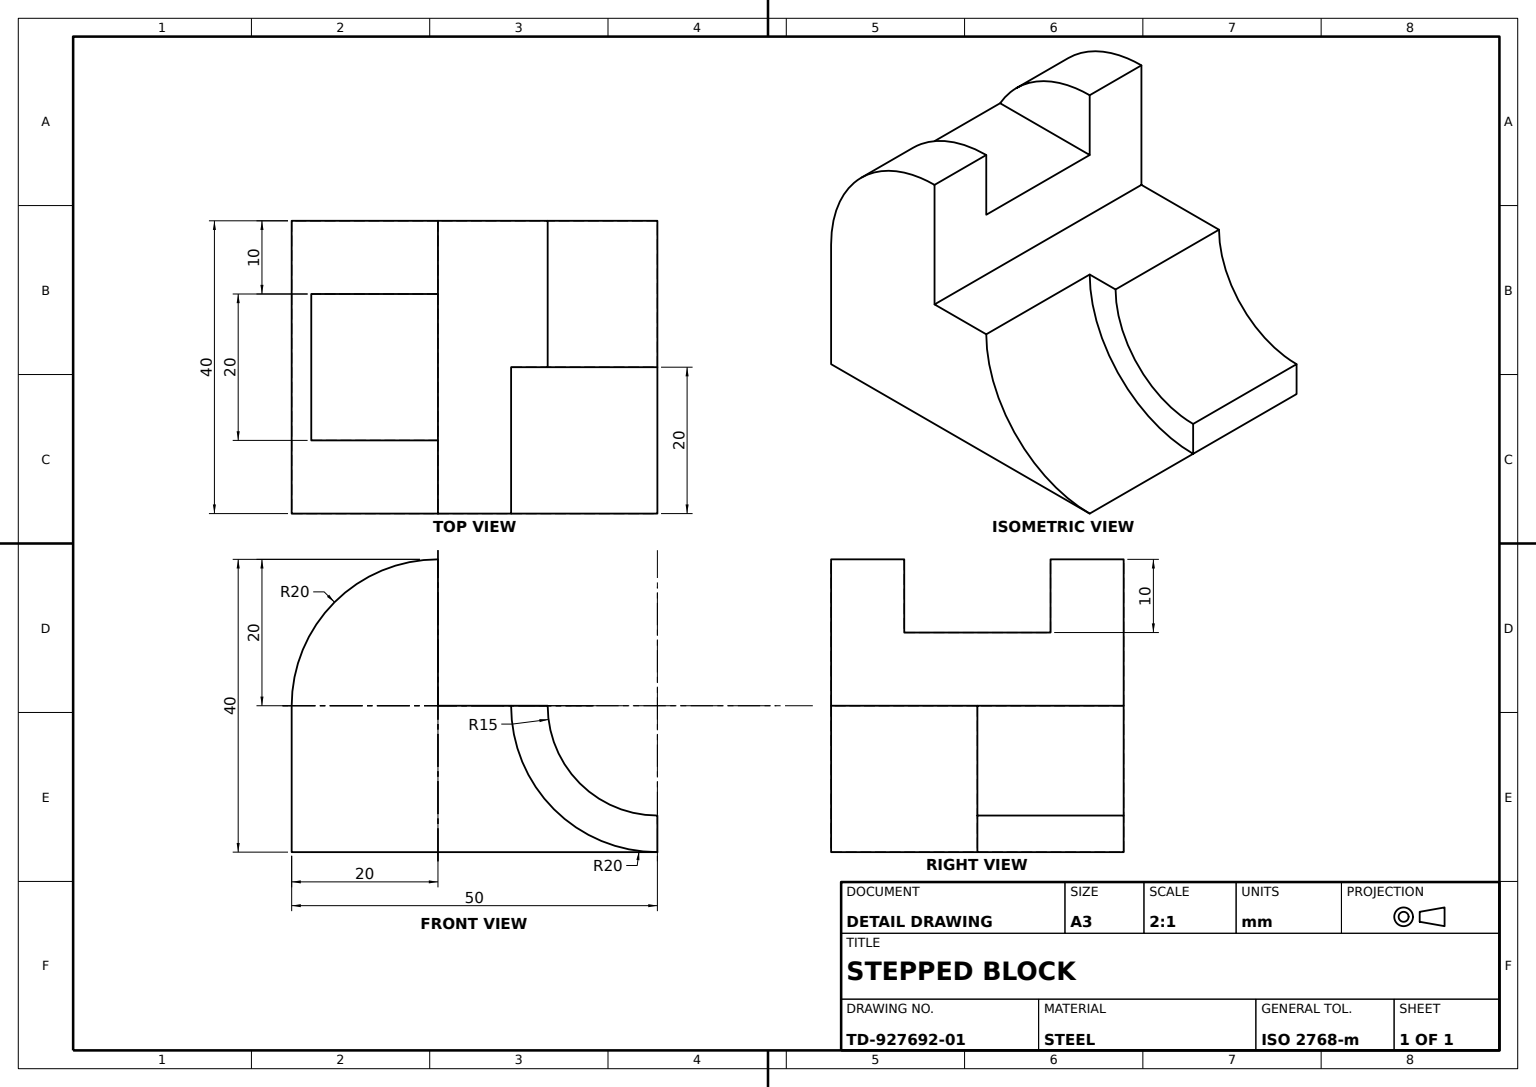
from build123d import *

# Parameters (mm, degrees)
BASE_BLOCK_PROFILE_W      = 50
BASE_BLOCK_PROFILE_H      = 40
BASE_BLOCK_50X40X40_DEPTH = 20
CORNER_NOTCH_PROFILE_W    = 20
CORNER_NOTCH_PROFILE_H    = 20
CORNER_NOTCH_20X20_DEPTH  = 76.498344353
STEP_CUT_DEPTH            = 20
CONCAVE_ARC_CUT_DEPTH     = 20
ARC_GROOVE_CUT_DEPTH      = 76.498344353
TOP_SLOT_PROFILE_10X10_W  = 20
TOP_SLOT_PROFILE_10X10_H  = 23.40818189
TOP_SLOT_10X10_DEPTH      = 20
ROUNDED_TOP_CUT_DEPTH     = 20
RIDGE_BOSS_PROFILE_W      = 20
RIDGE_BOSS_PROFILE_H      = 20
RIDGE_BOSS_10_DEPTH       = 10
RIDGE_ROUND_CUT_DEPTH     = 20


with BuildPart() as part:
    # Base Block Profile → Base Block 50x40x40 (new, symmetric)
    with BuildSketch(Plane.XY):
        with Locations((25, 20)):
            Rectangle(BASE_BLOCK_PROFILE_W, BASE_BLOCK_PROFILE_H)
    extrude(amount=BASE_BLOCK_50X40X40_DEPTH, both=True)

    # Corner Notch Profile → Corner Notch 20x20 (cut, through all)
    with BuildSketch(Plane.XY.offset(20)):
        with Locations((40, 30)):
            Rectangle(CORNER_NOTCH_PROFILE_W, CORNER_NOTCH_PROFILE_H)
    extrude(amount=-CORNER_NOTCH_20X20_DEPTH, mode=Mode.SUBTRACT)

    # Step Cut Profile → Step Cut (cut)
    with BuildSketch(Plane.XY.offset(20)):
        with BuildLine():
            Line((50, 0), (50, 20))
            Line((50, 20), (30, 20))
            ThreePointArc((30, 20), (35.857864376, 5.857864376), (50, 0))
        make_face()
    extrude(amount=-STEP_CUT_DEPTH, mode=Mode.SUBTRACT)

    # Concave Arc Profile R30 → Concave Arc Cut (cut)
    with BuildSketch(Plane.XY):
        with BuildLine():
            Line((50, 5), (50, 20))
            Line((50, 20), (35, 20))
            ThreePointArc((35, 20), (39.393398282, 9.393398282), (50, 5))
        make_face()
    extrude(amount=-CONCAVE_ARC_CUT_DEPTH, mode=Mode.SUBTRACT)

    # Arc Groove Profile → Arc Groove Cut (cut, through all)
    with BuildSketch(Plane.XY.offset(20)):
        with BuildLine():
            Line((0, 40), (0, 20))
            ThreePointArc((0, 20), (5.857864376, 34.142135624), (20, 40))
            Line((20, 40), (0, 40))
        make_face()
    extrude(amount=-ARC_GROOVE_CUT_DEPTH, mode=Mode.SUBTRACT)

    # Top Slot Profile 10x10 → Top Slot 10x10 (cut)
    with BuildSketch(Plane.ZY):
        with Locations((0, 31.704090945)):
            Rectangle(TOP_SLOT_PROFILE_10X10_W, TOP_SLOT_PROFILE_10X10_H)
    extrude(amount=-TOP_SLOT_10X10_DEPTH, mode=Mode.SUBTRACT)

    # Rounded Top Profile → Rounded Top Cut (cut)
    with BuildSketch(Plane(origin=(0, 40, 0), x_dir=(1, 0, 0), z_dir=(0, 1, 0))):
        Polygon((20, 20), (20, 10), (20, -10), (20, -20), (30, -20), (30, 20), align=None)
    extrude(amount=-ROUNDED_TOP_CUT_DEPTH, mode=Mode.SUBTRACT)

    # Ridge Boss Profile → Ridge Boss 10 (add)
    with BuildSketch(Plane(origin=(0, 20, 0), x_dir=(1, 0, 0), z_dir=(0, 1, 0))):
        with Locations((10, 0)):
            Rectangle(RIDGE_BOSS_PROFILE_W, RIDGE_BOSS_PROFILE_H)
    extrude(amount=RIDGE_BOSS_10_DEPTH)

    # Ridge Round Profile → Ridge Round Cut (cut)
    with BuildSketch(Plane.XY.offset(10)):
        with BuildLine():
            Line((0, 30), (0, 20))
            ThreePointArc((0, 20), (0.681483474, 25.176380902), (2.679491924, 30))
            Line((2.679491924, 30), (0, 30))
        make_face()
    extrude(amount=-RIDGE_ROUND_CUT_DEPTH, mode=Mode.SUBTRACT)


solid = part.part
